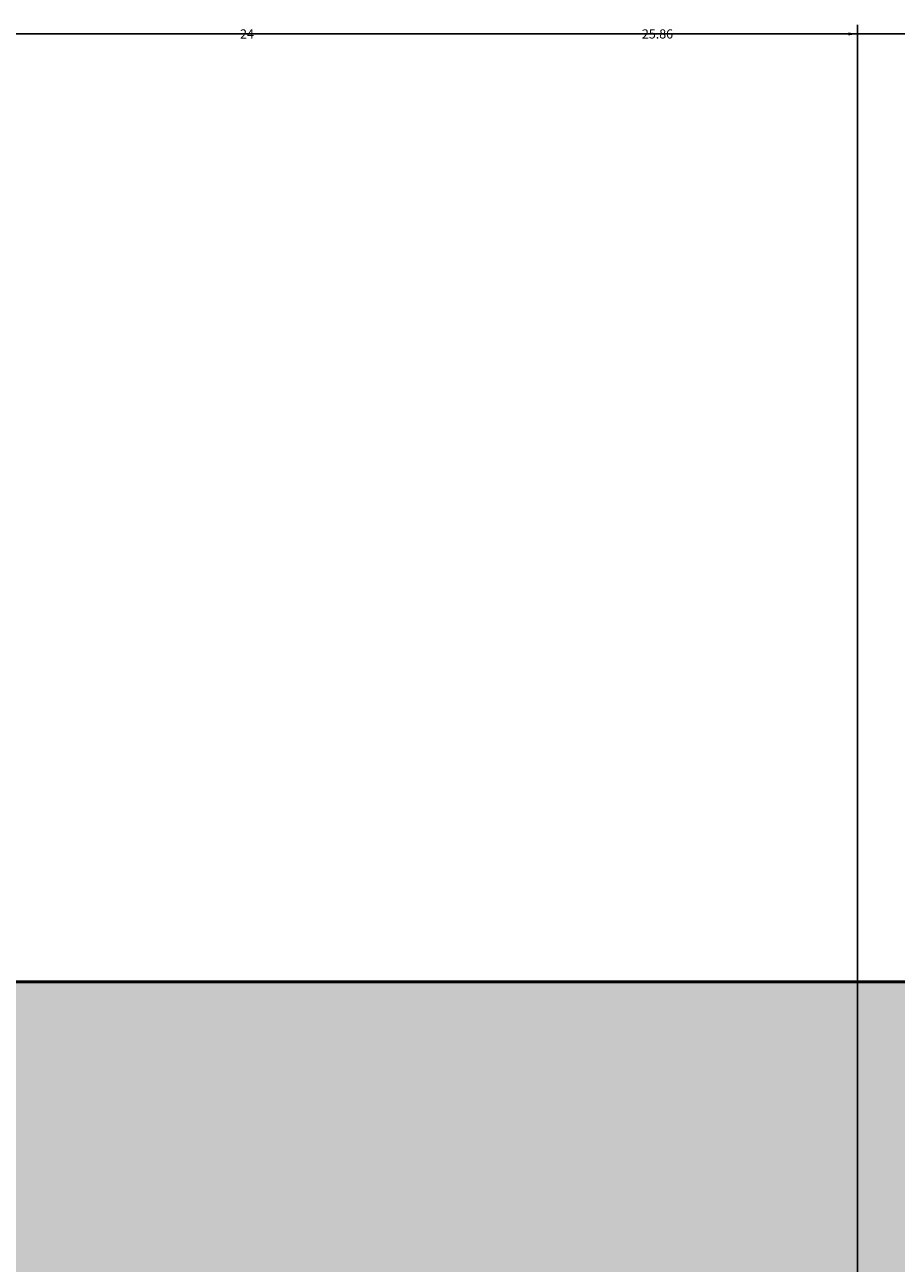
# Model space of a CAD drawing. Units: inches. Extents: x 2231 to 2461, y 2045 to 2455.
# Tile 94 of 95: x 2416 to 2434, y 2430 to 2455. Entities that reach past the tile are written whole.
import ezdxf

# ---------------------------------------------------------------- set-up
doc = ezdxf.new("R2010")
doc.units = ezdxf.units.IN
doc.layers.add('A-ANNO-DIMS', color=2, linetype='Continuous', lineweight=18)
doc.layers.add('A-WALL', color=7, linetype='Continuous', lineweight=50)
doc.layers.add('A-WALL-PATT', color=18, linetype='Continuous', lineweight=13, true_color=0x000000)
doc.styles.get("Standard").update_dxf_attribs({"font": 'arial.ttf'})
doc.dimstyles.get("Standard").update_dxf_attribs({"dimtxt": 0.18, "dimasz": 0.18, "dimexe": 0.18, "dimexo": 0.0625, "dimgap": 0.09, "dimtad": 0, "dimtih": 1, "dimtoh": 1, "dimdec": 4, "dimzin": 0, "dimdsep": 46, "dimtxsty": 'Standard', "dimcen": 0.09, "dimadec": 0, "dimazin": 0, "dimtfac": 1, "dimtdec": 4, "dimtofl": 0, "dimtmove": 0, "dimatfit": 3, "dimfxl": 1, "dimtolj": 1, "dimtzin": 0, "dimarcsym": 0})

# ---------------------------------------------------------------- blocks, each defined once
blk = doc.blocks.new('*D36')
at = {"layer": 'A-ANNO-DIMS', "color": 0, "lineweight": -2, "transparency": 16777216}
for p, q in [((2372.794, 2426.895), (2372.794, 2454.645)), ((2432.794, 2426.895), (2432.794, 2454.645)), ((2372.974, 2454.465), (2402.574, 2454.465)), ((2432.614, 2454.465), (2403.013, 2454.465))]:
    blk.add_line(p, q, dxfattribs=at)
at = {"layer": 'A-ANNO-DIMS', "color": 0, "transparency": 16777216}
for points in [[(2372.974, 2454.495), (2372.974, 2454.435), (2372.794, 2454.465)], [(2432.614, 2454.495), (2432.614, 2454.435), (2432.794, 2454.465)]]:
    blk.add_solid(points, dxfattribs=at)
at = {"layer": 'Defpoints', "color": 0, "transparency": 16777216}
for p in [(2432.794, 2454.465), (2372.794, 2426.833), (2432.794, 2426.833)]:
    blk.add_point(p, dxfattribs=at)
at = {"layer": 'A-ANNO-DIMS', "color": 0, "transparency": 16777216, "insert": (2402.794, 2454.465), "char_height": 0.18, "attachment_point": 5}
blk.add_mtext('\\A1;60', dxfattribs=at)
blk = doc.blocks.new('*D42')
at = {"layer": 'A-ANNO-DIMS', "color": 0, "lineweight": -2, "transparency": 16777216}
for p, q in [((2396.794, 2286.895), (2396.794, 2454.645)), ((2432.794, 2286.895), (2432.794, 2454.645)), ((2396.974, 2454.465), (2414.575, 2454.465)), ((2432.614, 2454.465), (2415.012, 2454.465))]:
    blk.add_line(p, q, dxfattribs=at)
at = {"layer": 'A-ANNO-DIMS', "color": 0, "transparency": 16777216}
for points in [[(2396.974, 2454.495), (2396.974, 2454.435), (2396.794, 2454.465)], [(2432.614, 2454.495), (2432.614, 2454.435), (2432.794, 2454.465)]]:
    blk.add_solid(points, dxfattribs=at)
at = {"layer": 'Defpoints', "color": 0, "transparency": 16777216}
for p in [(2432.794, 2454.465), (2396.794, 2286.833), (2432.794, 2286.833)]:
    blk.add_point(p, dxfattribs=at)
at = {"layer": 'A-ANNO-DIMS', "color": 0, "transparency": 16777216, "insert": (2414.794, 2454.465), "char_height": 0.18, "attachment_point": 5}
blk.add_mtext('\\A1;36', dxfattribs=at)
blk = doc.blocks.new('*D56')
at = {"layer": 'A-ANNO-DIMS', "color": 0, "lineweight": -2, "transparency": 16777216}
for p, q in [((2415.934, 2435.895), (2415.934, 2454.645)), ((2441.794, 2435.895), (2441.794, 2454.645)), ((2416.114, 2454.465), (2428.468, 2454.465)), ((2441.614, 2454.465), (2429.259, 2454.465))]:
    blk.add_line(p, q, dxfattribs=at)
at = {"layer": 'A-ANNO-DIMS', "color": 0, "transparency": 16777216}
for points in [[(2416.114, 2454.495), (2416.114, 2454.435), (2415.934, 2454.465)], [(2441.614, 2454.495), (2441.614, 2454.435), (2441.794, 2454.465)]]:
    blk.add_solid(points, dxfattribs=at)
at = {"layer": 'Defpoints', "color": 0, "transparency": 16777216}
for p in [(2441.794, 2454.465), (2415.934, 2435.833), (2441.794, 2435.833)]:
    blk.add_point(p, dxfattribs=at)
at = {"layer": 'A-ANNO-DIMS', "color": 0, "transparency": 16777216, "insert": (2428.864, 2454.465), "char_height": 0.18, "attachment_point": 5}
blk.add_mtext('\\A1;25.86', dxfattribs=at)
blk = doc.blocks.new('*D59')
at = {"layer": 'A-ANNO-DIMS', "color": 0, "lineweight": -2, "transparency": 16777216}
for p, q in [((2408.794, 2182.895), (2408.794, 2454.645)), ((2432.794, 2182.895), (2432.794, 2454.645)), ((2408.974, 2454.465), (2420.573, 2454.465)), ((2432.614, 2454.465), (2421.014, 2454.465))]:
    blk.add_line(p, q, dxfattribs=at)
at = {"layer": 'A-ANNO-DIMS', "color": 0, "transparency": 16777216}
for points in [[(2408.974, 2454.495), (2408.974, 2454.435), (2408.794, 2454.465)], [(2432.614, 2454.495), (2432.614, 2454.435), (2432.794, 2454.465)]]:
    blk.add_solid(points, dxfattribs=at)
at = {"layer": 'Defpoints', "color": 0, "transparency": 16777216}
for p in [(2432.794, 2454.465), (2408.794, 2182.833), (2432.794, 2182.833)]:
    blk.add_point(p, dxfattribs=at)
at = {"layer": 'A-ANNO-DIMS', "color": 0, "transparency": 16777216, "insert": (2420.794, 2454.465), "char_height": 0.18, "attachment_point": 5}
blk.add_mtext('\\A1;24', dxfattribs=at)

msp = doc.modelspace()

# ---------------------------------------------------------------- hatches: boundary and pattern name
at = {"layer": 'A-WALL-PATT'}
h = msp.add_hatch(color=256, dxfattribs=at)
h.dxf.hatch_style = 1
h.paths.add_polyline_path([(2441.7935, 2269.1535), (2432.7935, 2269.1535), (2432.7935, 2186.8328), (2396.7935, 2186.8328), (2396.7935, 2286.8328), (2394.7935, 2286.8328), (2394.7935, 2186.8328), (2334.7935, 2186.8328), (2334.7935, 2182.8328), (2432.7935, 2182.8328), (2432.7935, 2072.8328), (2416.6639, 2072.8328), (2416.6639, 2063.8328), (2441.7935, 2063.8328)])
h.paths.add_polyline_path([(2368.6639, 2072.8328), (2367.04, 2072.8328), (2330.7942, 2072.8328), (2330.7397, 2063.8328), (2368.6639, 2063.8328)])
h.paths.add_polyline_path([(2300.7392, 2068.3328), (2300.7392, 2072.8328), (2298.7935, 2072.8328), (2294.7935, 2072.8328), (2258.7935, 2072.8328), (2258.7935, 2120.8328), (2294.7935, 2120.8328), (2298.7935, 2120.8328), (2298.7935, 2128.8328), (2294.7935, 2128.8328), (2294.7935, 2124.8328), (2258.7935, 2124.8328), (2258.7935, 2182.8328), (2294.7935, 2182.8328), (2294.7935, 2174.8328), (2298.7935, 2174.8328), (2298.7935, 2182.8328), (2304.7935, 2182.8328), (2304.7935, 2186.8328), (2258.7935, 2186.8328), (2258.7935, 2221.999), (2249.7935, 2221.999), (2249.7935, 2063.8328), (2300.7392, 2063.8328)])
h.paths.add_polyline_path([(2391.9338, 2435.8328), (2333.82, 2435.8328), (2333.82, 2426.8328), (2368.7935, 2426.8328), (2368.7935, 2374.9508), (2368.7935, 2370.8328), (2372.3935, 2370.8328), (2372.7935, 2370.8328), (2372.7935, 2426.8328), (2391.9338, 2426.8328)])
h.paths.add_polyline_path([(2441.7935, 2435.8328), (2415.9338, 2435.8328), (2415.9338, 2426.8328), (2432.7935, 2426.8328), (2432.7935, 2334.8328), (2372.7935, 2334.8328), (2372.7935, 2346.8328), (2368.7935, 2346.8328), (2368.7935, 2306.8328), (2360.7935, 2306.8328), (2360.7935, 2302.8328), (2368.7935, 2302.8328), (2372.7935, 2302.8328), (2372.7935, 2330.8328), (2432.7935, 2330.8328), (2432.7935, 2317.1535), (2441.7935, 2317.1535)])
h.paths.add_polyline_path([(2285.82, 2435.8328), (2249.7935, 2435.8328), (2249.7935, 2269.999), (2258.7935, 2269.999), (2258.7935, 2302.8328), (2318.8168, 2302.8328), (2330.7935, 2302.8328), (2330.7935, 2306.8328), (2258.7935, 2306.8328), (2258.7935, 2426.8328), (2285.82, 2426.8328)])

# ---------------------------------------------------------------- linework, layer by layer
at = {"layer": 'A-WALL'}
msp.add_lwpolyline([(2300.7392, 2063.8328), (2249.7935, 2063.8328), (2249.7935, 2435.8328), (2441.7935, 2435.8328), (2441.7935, 2063.8328), (2330.7397, 2063.8328)], dxfattribs=at)

# ---------------------------------------------------------------- dimensions: what is measured, and where the dimension line sits
at = {"layer": 'A-ANNO-DIMS'}
for base, p1, p2, override, picture, middle in [((2432.7935, 2454.4653), (2372.7935, 2426.8328), (2432.7935, 2426.8328), {"dimdec": 0, "dimlfac": 1, "dimrnd": 0, "dimzin": 0, "dimdsep": 46, "dimlunit": 2}, '*D36', (2402.7935, 2454.4653)), ((2432.7935, 2454.4653), (2396.7935, 2286.8328), (2432.7935, 2286.8328), {"dimdec": 0, "dimlfac": 1, "dimrnd": 0, "dimzin": 0, "dimdsep": 46, "dimlunit": 2}, '*D42', (2414.7935, 2454.4653)), ((2432.7935, 2454.4653), (2408.7935, 2182.8328), (2432.7935, 2182.8328), {"dimdec": 0, "dimlfac": 1, "dimrnd": 0, "dimzin": 0, "dimdsep": 46, "dimlunit": 2}, '*D59', (2420.7935, 2454.4653)), ((2441.7935, 2454.4653), (2415.9338, 2435.8328), (2441.7935, 2435.8328), {"dimdec": 2, "dimlfac": 1, "dimrnd": 0, "dimzin": 0, "dimdsep": 46, "dimlunit": 2}, '*D56', (2428.8637, 2454.4653))]:
    dim = msp.add_linear_dim(base=base, p1=p1, p2=p2, dimstyle='Standard', override=override, dxfattribs=at)
    dim.commit()
    dim.dimension.update_dxf_attribs({"geometry": picture, "text_midpoint": middle})

doc.saveas('drawing.dxf')
